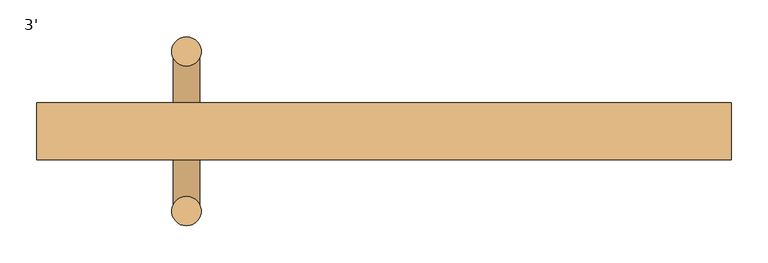
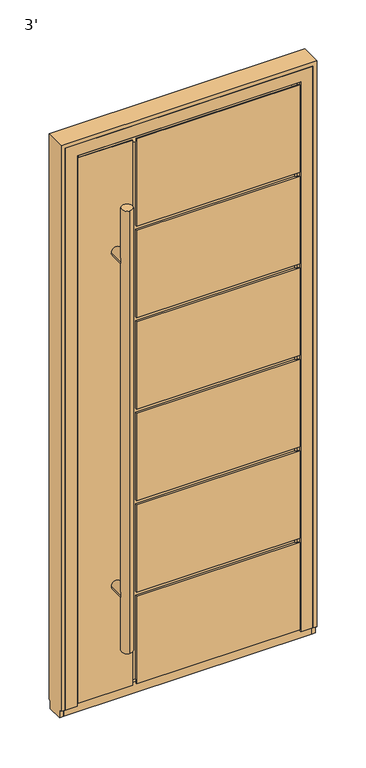
"""IFC4 building model written with IfcOpenShell, lengths in millimetres: door geometry, 3'."""

from ifc_helpers import new_model, si_unit, point, frame, frame_2d, origin, place, context, project, spatial, circle_curve, trimmed, segment, composite_curve, outline, extrude, faceted_brep, source, transform, mapped, element, save


def door_3_130b8d4e(model_context):
    return source(origin(), model_context, "Body", "SolidModel", [
        extrude(outline(composite_curve([segment(trimmed(circle_curve(frame_2d((-268.65, 52.7003001)), 20.0), [point((-268.65, 32.7003001))], [point((-268.65, 72.7003001))], False, "CARTESIAN"), True, "CONTINUOUS"), segment(trimmed(circle_curve(frame_2d((-268.65, 52.7003001)), 20.0), [point((-268.65, 72.7003001))], [point((-268.65, 32.7003001))], False, "CARTESIAN"), True, "CONTINUOUS")], self_intersect=False)), frame((0.0, 0.0, 210.0000003), z_axis=(0.0, 0.0, 1.0), x_axis=(1.0, 0.0, 0.0)), (0.0, 0.0, 1.0), 1724.5),
        extrude(outline(composite_curve([segment(trimmed(circle_curve(frame_2d((-268.65, -164.3003001)), 20.0), [point((-268.65, -184.3003001))], [point((-268.65, -144.3003001))], False, "CARTESIAN"), True, "CONTINUOUS"), segment(trimmed(circle_curve(frame_2d((-268.65, -164.3003001)), 20.0), [point((-268.65, -144.3003001))], [point((-268.65, -184.3003001))], False, "CARTESIAN"), True, "CONTINUOUS")], self_intersect=False)), frame((0.0, 0.0, 210.0000003), z_axis=(0.0, 0.0, 1.0), x_axis=(1.0, 0.0, 0.0)), (0.0, 0.0, 1.0), 1724.5),
        extrude(outline(composite_curve([segment(trimmed(circle_curve(frame_2d((422.2500003, -268.65)), 18.0), [point((422.2500003, -286.65))], [point((422.2500003, -250.65))], False, "CARTESIAN"), True, "CONTINUOUS"), segment(trimmed(circle_curve(frame_2d((422.2500003, -268.65)), 18.0), [point((422.2500003, -250.65))], [point((422.2500003, -286.65))], False, "CARTESIAN"), True, "CONTINUOUS")], self_intersect=False)), frame((0.0, -164.3, 0.0), z_axis=(0.0, 1.0, 0.0), x_axis=(0.0, 0.0, 1.0)), (0.0, 0.0, 1.0), 217.0),
        extrude(outline(composite_curve([segment(trimmed(circle_curve(frame_2d((1722.2500003, -268.65)), 18.0), [point((1722.2500003, -286.65))], [point((1722.2500003, -250.65))], False, "CARTESIAN"), True, "CONTINUOUS"), segment(trimmed(circle_curve(frame_2d((1722.2500003, -268.65)), 18.0), [point((1722.2500003, -250.65))], [point((1722.2500003, -286.65))], False, "CARTESIAN"), True, "CONTINUOUS")], self_intersect=False)), frame((0.0, -164.3, 0.0), z_axis=(0.0, 1.0, 0.0), x_axis=(0.0, 0.0, 1.0)), (0.0, 0.0, 1.0), 217.0),
        faceted_brep([(-193.65, -24.3, 366.5833337), (383.65, -24.3, 366.5833337), (383.65, -24.3, 351.5833337), (-193.65, -24.3, 351.5833337), (-193.65, -24.3, 35.0), (-208.65, -24.3, 35.0), (-208.65, -24.3, 2109.5000003), (-193.65, -24.3, 2109.5000003), (-193.65, -24.3, 1792.916667), (383.65, -24.3, 1792.916667), (383.65, -24.3, 1777.916667), (-193.65, -24.3, 1777.916667), (-193.65, -24.3, 1436.3333337), (383.65, -24.3, 1436.3333337), (383.65, -24.3, 1421.3333337), (-193.65, -24.3, 1421.3333337), (-193.65, -24.3, 1079.7500004), (383.65, -24.3, 1079.7500004), (383.65, -24.3, 1064.7500004), (-193.65, -24.3, 1064.7500004), (-193.65, -24.3, 723.166667), (383.65, -24.3, 723.166667), (383.65, -24.3, 708.166667), (-193.65, -24.3, 708.166667), (-193.65, -17.3, 708.166667), (-193.65, -17.3, 366.5833337), (383.65, -17.3, 708.166667), (383.65, -26.3002302, 2109.5000003), (383.65, -26.3002302, 35.0), (383.65, -19.2979528, 35.0), (383.65, -19.2979528, 24.0), (383.65, -17.3, 24.0), (383.65, -17.3, 351.5833337), (383.65, -17.3, 366.5833337), (383.65, -17.3, 723.166667), (383.65, -17.3, 1064.7500004), (383.65, -17.3, 1079.7500004), (383.65, -17.3, 1421.3333337), (383.65, -17.3, 1436.3333337), (383.65, -17.3, 1777.916667), (383.65, -17.3, 1792.916667), (383.65, -17.3, 2109.5000003), (-193.65, -17.3, 723.166667), (-193.65, -17.3, 1064.7500004), (-193.65, -17.3, 1079.7500004), (-193.65, -17.3, 1421.3333337), (-208.65, -19.2979528, 35.0), (-208.65, -19.2979528, 24.0), (-208.65, -17.3, 24.0), (-208.65, -17.3, 2109.5000003), (-383.65, -26.3002302, 35.0), (-383.65, -19.2979528, 35.0), (-193.65, -19.2979528, 35.0), (-193.65, -17.3, 351.5833337), (-193.65, -17.3, 24.0), (-193.65, -19.2979528, 24.0), (-383.65, -19.2979528, 24.0), (-383.65, -17.3, 24.0), (-383.65, -17.3, 2109.5000003), (-193.65, -17.3, 1436.3333337), (-193.65, -17.3, 1777.916667), (-193.65, -17.3, 1792.916667), (-193.65, -17.3, 2109.5000003), (408.65, -94.3, 10.0000003), (-193.65, -94.3, 10.0000003), (-193.65, -91.3, 10.0000003), (408.65, -91.3, 10.0000003), (-408.65, -91.3, 10.0000003), (-208.65, -91.3, 10.0000003), (-208.65, -94.3, 10.0000003), (-408.65, -94.3, 10.0000003), (408.65, -94.3, 366.5833337), (408.65, -91.3, 366.5833337), (408.65, -91.3, 708.166667), (408.65, -94.3, 708.166667), (408.65, -94.3, 1079.7500004), (408.65, -91.3, 1079.7500004), (408.65, -91.3, 1421.3333337), (408.65, -94.3, 1421.3333337), (408.65, -94.3, 723.166667), (408.65, -91.3, 723.166667), (408.65, -91.3, 1064.7500004), (408.65, -94.3, 1064.7500004), (408.65, -94.3, 1436.3333337), (408.65, -91.3, 1436.3333337), (408.65, -91.3, 1777.916667), (408.65, -94.3, 1777.916667), (408.65, -94.3, 2134.5000003), (408.65, -94.3, 1792.916667), (408.65, -91.3, 1792.916667), (408.65, -91.3, 2134.5000003), (408.65, -91.3, 351.5833337), (408.65, -94.3, 351.5833337), (-193.65, -91.3, 25.5), (393.15, -91.3, 25.5), (393.15, -91.3, 351.5833337), (393.15, -91.3, 366.5833337), (393.15, -91.3, 708.166667), (393.15, -91.3, 1079.7500004), (393.15, -91.3, 1421.3333337), (393.15, -91.3, 723.166667), (393.15, -91.3, 1064.7500004), (-393.15, -91.3, 25.5), (-208.65, -91.3, 25.5), (-408.65, -91.3, 2134.5000003), (-208.65, -91.3, 2134.5000003), (-208.65, -91.3, 2119.0000003), (-393.15, -91.3, 2119.0000003), (393.15, -91.3, 1436.3333337), (393.15, -91.3, 1777.916667), (393.15, -91.3, 1792.916667), (393.15, -91.3, 2119.0000003), (-193.65, -91.3, 2119.0000003), (-193.65, -91.3, 2134.5000003), (-193.65, -87.3, 351.5833337), (-193.65, -87.3, 25.5), (-193.65, -94.3, 351.5833337), (-208.65, -94.3, 2134.5000003), (-408.65, -94.3, 2134.5000003), (-193.65, -94.3, 708.166667), (-193.65, -94.3, 366.5833337), (-193.65, -94.3, 1421.3333337), (-193.65, -94.3, 1079.7500004), (-193.65, -94.3, 1064.7500004), (-193.65, -94.3, 723.166667), (-193.65, -94.3, 1777.916667), (-193.65, -94.3, 1436.3333337), (-193.65, -94.3, 2134.5000003), (-193.65, -94.3, 1792.916667), (-208.65, -87.3, 2119.0000003), (-208.65, -87.3, 25.5), (-383.65, -26.3002302, 2109.5000003), (393.15, -26.3002302, 2119.0000003), (393.15, -26.3002302, 25.5), (-393.15, -26.3002302, 25.5), (-393.15, -26.3002302, 2119.0000003), (393.15, -87.3, 1792.916667), (393.15, -87.3, 1777.916667), (393.15, -87.3, 1436.3333337), (393.15, -87.3, 1421.3333337), (393.15, -87.3, 1079.7500004), (393.15, -87.3, 1064.7500004), (393.15, -87.3, 723.166667), (393.15, -87.3, 708.166667), (393.15, -87.3, 366.5833337), (393.15, -87.3, 351.5833337), (-193.65, -87.3, 1777.916667), (-193.65, -87.3, 1792.916667), (-193.65, -87.3, 2119.0000003), (-193.65, -87.3, 366.5833337), (-193.65, -87.3, 708.166667), (-193.65, -87.3, 723.166667), (-193.65, -87.3, 1064.7500004), (-193.65, -87.3, 1079.7500004), (-193.65, -87.3, 1421.3333337), (-193.65, -87.3, 1436.3333337)], [[[0, 1, 2, 3, 4, 5, 6, 7, 8, 9, 10, 11, 12, 13, 14, 15, 16, 17, 18, 19, 20, 21, 22, 23]], [[23, 24, 25, 0]], [[23, 22, 26, 24]], [[27, 28, 29, 30, 31, 32, 2, 1, 33, 26, 22, 21, 34, 35, 18, 17, 36, 37, 14, 13, 38, 39, 10, 9, 40, 41]], [[42, 34, 21, 20]], [[19, 43, 42, 20]], [[19, 18, 35, 43]], [[44, 36, 17, 16]], [[15, 45, 44, 16]], [[5, 46, 47, 48, 49, 6]], [[28, 50, 51, 46, 5, 4, 52, 29]], [[53, 54, 55, 52, 4, 3]], [[3, 2, 32, 53]], [[25, 33, 1, 0]], [[29, 52, 55, 30]], [[56, 47, 46, 51]], [[30, 55, 54, 31]], [[57, 48, 47, 56]], [[36, 44, 45, 37]], [[34, 42, 43, 35]], [[33, 25, 24, 26]], [[54, 53, 32, 31]], [[58, 49, 48, 57]], [[38, 59, 60, 39]], [[41, 40, 61, 62]], [[63, 64, 65, 66]], [[67, 68, 69, 70]], [[71, 72, 73, 74]], [[75, 76, 77, 78]], [[79, 80, 81, 82]], [[83, 84, 85, 86]], [[87, 88, 89, 90]], [[66, 91, 92, 63]], [[65, 93, 94, 95, 91, 66]], [[72, 96, 97, 73]], [[76, 98, 99, 77]], [[80, 100, 101, 81]], [[102, 103, 68, 67, 104, 105, 106, 107]], [[84, 108, 109, 85]], [[90, 89, 110, 111, 112, 113]], [[114, 115, 93, 65, 64, 116]], [[70, 69, 117, 118]], [[63, 92, 116, 64]], [[74, 119, 120, 71]], [[78, 121, 122, 75]], [[82, 123, 124, 79]], [[86, 125, 126, 83]], [[87, 127, 128, 88]], [[70, 118, 104, 67]], [[129, 106, 105, 117, 69, 68, 103, 130]], [[58, 57, 56, 51, 50, 131]], [[132, 133, 134, 135], [131, 50, 28, 27]], [[111, 110, 136, 137, 109, 108, 138, 139, 99, 98, 140, 141, 101, 100, 142, 143, 97, 96, 144, 145, 95, 94, 133, 132]], [[94, 93, 115, 130, 103, 102, 134, 133]], [[135, 134, 102, 107]], [[146, 137, 136, 147, 148, 129, 130, 115, 114, 145, 144, 149, 150, 143, 142, 151, 152, 141, 140, 153, 154, 139, 138, 155]], [[153, 122, 121, 154]], [[153, 140, 98, 76, 75, 122]], [[123, 82, 81, 101, 141, 152]], [[151, 124, 123, 152]], [[151, 142, 100, 80, 79, 124]], [[119, 74, 73, 97, 143, 150]], [[149, 120, 119, 150]], [[149, 144, 96, 72, 71, 120]], [[116, 92, 91, 95, 145, 114]], [[15, 14, 37, 45]], [[59, 38, 13, 12]], [[11, 60, 59, 12]], [[11, 10, 39, 60]], [[61, 40, 9, 8]], [[8, 7, 62, 61]], [[125, 86, 85, 109, 137, 146]], [[128, 127, 113, 112, 148, 147]], [[121, 78, 77, 99, 139, 154]], [[155, 138, 108, 84, 83, 126]], [[155, 126, 125, 146]], [[147, 136, 110, 89, 88, 128]], [[90, 113, 127, 87]], [[118, 117, 105, 104]], [[132, 135, 107, 106, 129, 148, 112, 111]], [[27, 41, 62, 7, 6, 49, 58, 131]]]),
        faceted_brep([(-457.2, -94.3, 0.0), (-457.2, -85.2997571, 0.0), (-412.7, -85.2997571, 0.0), (-412.7, -94.3, 0.0), (-403.2, -21.8000042, 0.0), (-403.2, -26.3, 0.0), (-457.2, -26.3, 0.0), (-457.2, -17.3, 0.0), (-387.7, -17.3, 0.0), (-387.7, -21.8000042, 0.0), (457.2, -17.3, 0.0), (457.2, -26.3, 0.0), (403.2, -26.3, 0.0), (403.2, -21.8000042, 0.0), (387.7, -21.8000042, 0.0), (387.7, -17.3, 0.0), (412.7, -85.2997571, 0.0), (457.2, -85.2997571, 0.0), (457.2, -94.3, 0.0), (412.7, -94.3, 0.0), (-457.2, -26.3, -30.0), (-457.2, -85.2997571, -30.0), (-457.2, -94.3, 2189.5), (-457.2, -17.3, 2189.5), (-412.7, -94.3, 2145.0), (412.7, -94.3, 2145.0), (457.2, -94.3, 2189.5), (457.2, -17.3, 2189.5), (457.2, -85.2997571, -30.0), (457.2, -26.3, -30.0), (387.7, -17.3, 2120.0), (-387.7, -17.3, 2120.0), (-403.2, -85.3, 2135.5), (-403.2, -85.3, 14.5), (-403.2, -26.3, 14.5), (-403.2, -21.8000042, 2135.5), (403.2, -21.8000042, 2135.5), (403.2, -85.3, 2135.5), (403.2, -26.3, 14.5), (403.2, -85.3, 14.5), (-412.7, -85.3, 2145.0), (412.7, -85.3, 2145.0), (-387.7, -21.8000042, 2120.0), (387.7, -21.8000042, 2120.0)], [[[0, 1, 2, 3]], [[4, 5, 6, 7, 8, 9]], [[10, 11, 12, 13, 14, 15]], [[16, 17, 18, 19]], [[7, 6, 20, 21, 1, 0, 22, 23]], [[3, 24, 25, 19, 18, 26, 22, 0]], [[22, 26, 27, 23]], [[18, 17, 28, 29, 11, 10, 27, 26]], [[7, 23, 27, 10, 15, 30, 31, 8]], [[32, 33, 34, 5, 4, 35]], [[35, 36, 37, 32]], [[36, 13, 12, 38, 39, 37]], [[40, 24, 3, 2]], [[16, 41, 40, 2, 1, 21, 28, 17], [37, 39, 33, 32]], [[9, 42, 43, 14, 13, 36, 35, 4]], [[8, 31, 42, 9]], [[24, 40, 41, 25]], [[30, 43, 42, 31]], [[19, 25, 41, 16]], [[14, 43, 30, 15]], [[20, 6, 5, 34, 38, 12, 11, 29]], [[39, 38, 34, 33]], [[20, 29, 28, 21]]]),
        faceted_brep([(-457.2, -85.3, -30.0), (-472.2, -85.3, -30.0), (-472.2, -26.3, -30.0), (-457.2, -26.3, -30.0), (-457.2, -94.3, 2189.5), (-457.2, -94.3, 0.0), (-457.2, -85.3, 0.0), (-457.2, -26.3, 0.0), (-457.2, -17.3, 0.0), (-457.2, -17.3, 2189.5), (-472.2, -26.3, 0.0), (472.2, -26.3, 0.0), (472.2, -26.3, -30.0), (457.2, -26.3, -30.0), (457.2, -26.3, 0.0), (-472.2, -17.3, 2204.5), (-472.2, -17.3, 0.0), (-472.2, -85.3, 0.0), (-472.2, -94.3, 0.0), (-472.2, -94.3, 2204.5), (457.2, -85.3, 0.0), (457.2, -85.3, -30.0), (472.2, -85.3, -30.0), (472.2, -85.3, 0.0), (457.2, -17.3, 2189.5), (457.2, -17.3, 0.0), (457.2, -94.3, 0.0), (457.2, -94.3, 2189.5), (472.2, -94.3, 0.0), (472.2, -94.3, 2204.5), (472.2, -17.3, 0.0), (472.2, -17.3, 2204.5)], [[[0, 1, 2, 3]], [[4, 5, 6, 0, 3, 7, 8, 9]], [[7, 3, 2, 10]], [[11, 12, 13, 14]], [[15, 16, 10, 2, 1, 17, 18, 19]], [[17, 1, 0, 6]], [[20, 21, 22, 23]], [[24, 25, 14, 13, 21, 20, 26, 27]], [[27, 26, 28, 29, 19, 18, 5, 4]], [[6, 5, 18, 17]], [[23, 28, 26, 20]], [[22, 21, 13, 12]], [[10, 16, 8, 7]], [[14, 25, 30, 11]], [[9, 8, 16, 15, 31, 30, 25, 24]], [[29, 28, 23, 22, 12, 11, 30, 31]], [[9, 24, 27, 4]], [[19, 29, 31, 15]]]),
    ])


if __name__ == "__main__":
    model = new_model("IFC4")
    model_context = context("Model", 3, world=origin())
    ifc_project = project(units=[si_unit("LENGTHUNIT", "METRE", prefix="MILLI")], contexts=[model_context])
    site = spatial("IfcSite", under=ifc_project)
    building = spatial("IfcBuilding", under=site)
    placement = place(None, origin())
    door_3_shape = door_3_130b8d4e(model_context)
    element("IfcDoor", 1, ObjectType="3'", at=placement, inside=building, context=model_context, shape_type="MappedRepresentation", body=[
        mapped(door_3_shape, transform((0.0, 0.0, 0.0), x_axis=(1.0, 0.0, 0.0), y_axis=(0.0, 1.0, 0.0), z_axis=(0.0, 0.0, 1.0))),
    ])
    save(model, "model.ifc")

# Revit data of these elements
# Type "3'"
#   Type Mark = "15"
#   Water resistance = "up to Class E900, EN 12208:2001"
#   Uniclass2015Version = "v1.21"
#   Uniclass2015Reference = "Ss_25_30_20_30"
#   Uniclass2015Description = "Frame and door leaf system"
#   URL = "www.aluprof.com"
#   Type IFC Predefined Type = "USERDEFINED"
#   Right-hand / Left-hand door [instance default] = ""
#   Resistance to wind load = "up to Class C5/B5, EN 12210:2001"
#   Insert type = "ST"
#   Hardware [instance default] = ""
#   Product page = "https://aluprof.com/en/architects/offer/window-and-door-systems/panel-doors#visualisation"
#   Operation = "SinglePanelOutwardOpening"
#   Opening type = "Outward"
#   NBSReference = "25-50-20/125"
#   NBSDescription = "Frame and door leaf system"
#   Important = "The actual acceptable construction dimensions are dependent on the selection of profiles and hardware, glazing type, construction weight and the construction’s operating conditions. These should be determined by a suitably qualified person, and using ALUPROF’s calculation software"
#   IfcExportType = "USERDEFINED"
#   IfcExportAs = "IfcDoorType"
#   Handle type [instance default] = ""
#   Manufacturer = "ALUPROF SA"
#   Export Type to IFC As = "IfcDoorType"
#   Door sill type [instance default] = ""
#   Description = "External single-leaf panel door outward opening"
#   Model = "MB-86 ST Panel Door AD07"
#   Content of the recyclate in the material = "69.2%"
#   COBie.Type.WarrantyDurationParts = ""
#   COBie.Type.Name = ""
#   COBie.Type.Manufacturer = "ALUPROF SA"
#   COBie.Space.Name = ""
#   COBie.Floor.Name = ""
#   COBie.Facility.Name = ""
#   COBie.CreatedOn = ""
#   COBie.Component.WarrantyStartDate = ""
#   COBie.Component.Name = "MB-86 ST Panel Door AD07"
#   Burglar resistance = "RC2"
#   Air permeability = "up to Class 4, EN 12207:2001"
#   Width of the active leaf = 2' - 8.17717"
#   Placement in wall = 0' - 0.7874"
#   Thickness = 0' - 3.0315"
#   Height of the opening sash = 6' - 11.64173"
#   Handle Offset = 3' - 5.33858"
#   Rough Height = 7' - 4.61024"
#   Rough Width = 3' - 1.1811"
#   Height = 7' - 2.20079"
#   Width = 3' - 0"
#   Construction depth = 0' - 3.0315"
#   Clear opening width = 2' - 3.94882"
#   Clear opening height = 6' - 10.67717"
#   Height of the array = 1' - 1.44816"
#   Schedule No. [instance default] = 1
#   Handrail [instance default] = yes
#   IsExternal = yes
#   Handle [instance default] = no
#   Door closer [instance default] = no
#   Function = 1
#   COBie.Type = yes
#   COBie = yes
#   Access control [instance default] = no
#   Panel = element 387710
#   Wall Closure = (empty or 0)
